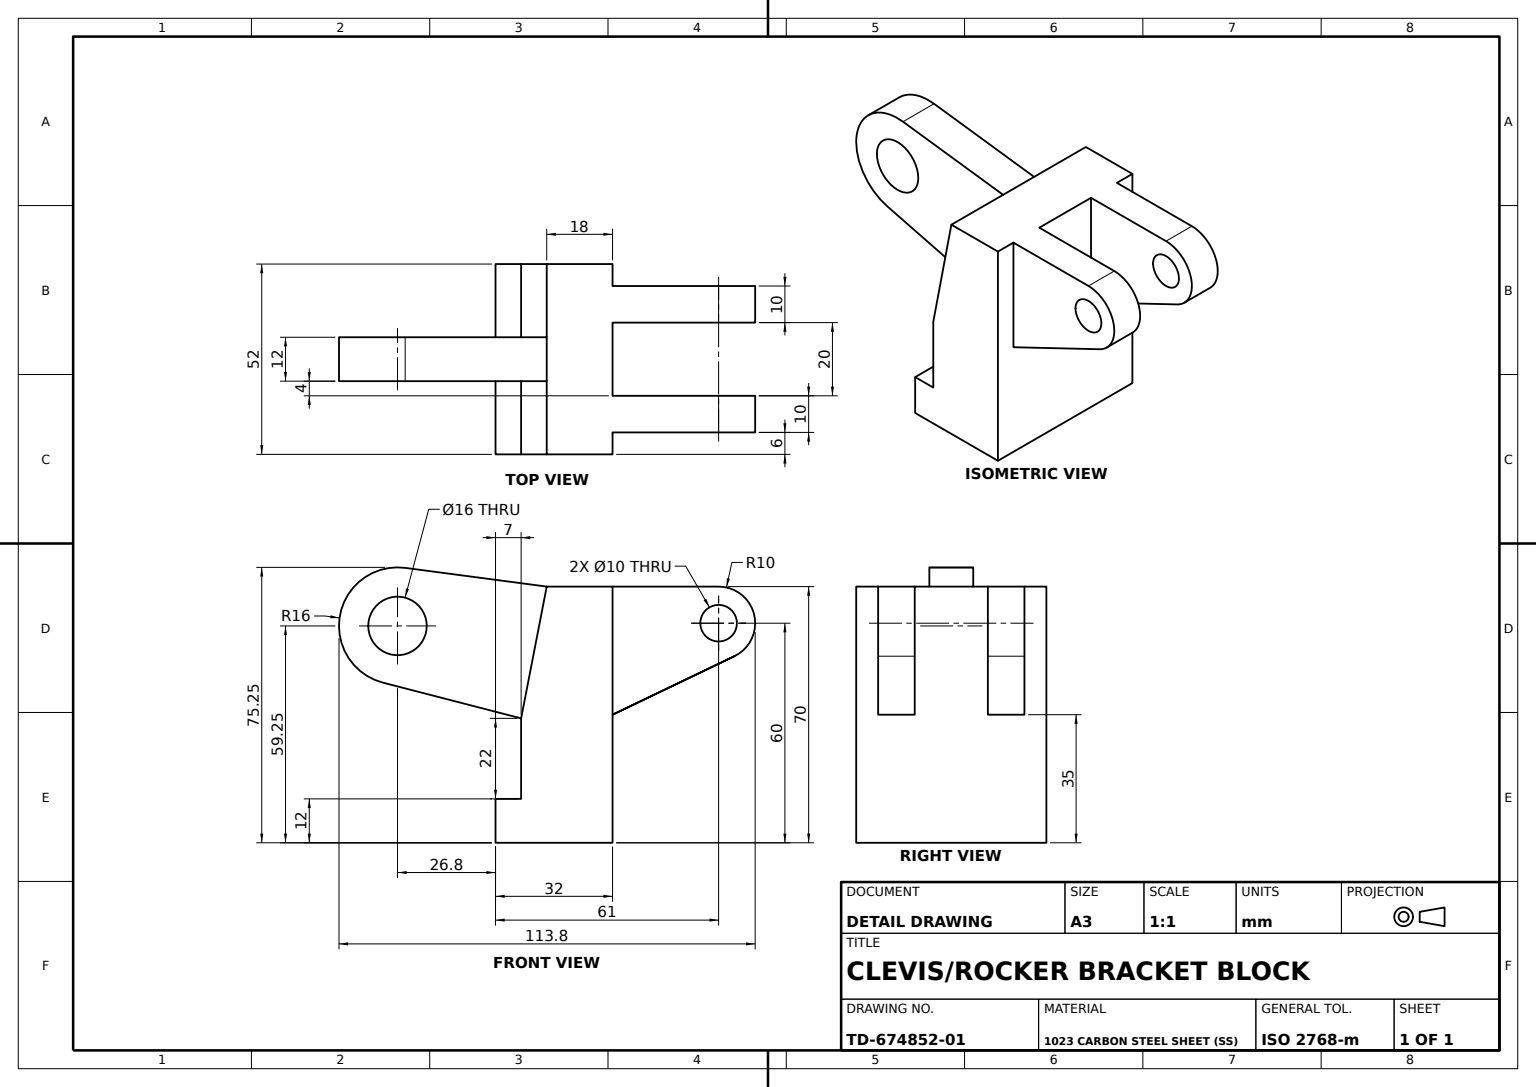
from build123d import *

# Parameters (mm, degrees)
BASE_BLOCK_SKETCH_W = 32
BASE_BLOCK_SKETCH_H = 12
BASE_BLOCK_DEPTH    = 52
UPRIGHT_BODY_DEPTH  = 52
CLEVIS_LUG_SKETCH_R = 5
CLEVIS_LUG_DEPTH    = 10
PIVOT_ARM_SKETCH_R  = 8
PIVOT_ARM_DEPTH     = 6


with BuildPart() as part:
    # Base Block Sketch → Base Block (new body)
    with BuildSketch(Plane.XY):
        with Locations((16, 6)):
            Rectangle(BASE_BLOCK_SKETCH_W, BASE_BLOCK_SKETCH_H)
    extrude(amount=BASE_BLOCK_DEPTH)

    # Upright Profile Sketch → Upright Body (add)
    with BuildSketch(Plane.XY.offset(52)):
        Polygon((32, 12), (32, 70), (14, 70), (7, 34), (7, 12), align=None)
    extrude(amount=-UPRIGHT_BODY_DEPTH)

    # Clevis Lug Sketch → Clevis Lug (add)
    with BuildSketch(Plane.XY.offset(6)):
        with BuildLine():
            Line((32, 70), (61, 70))
            ThreePointArc((61, 70), (70.751033946, 62.217506931), (65.324597071, 50.983467397))
            Line((65.324597071, 50.983467397), (32, 35))
            Line((32, 35), (32, 70))
        make_face()
        with Locations((61, 60)):
            Circle(CLEVIS_LUG_SKETCH_R, mode=Mode.SUBTRACT)
    clevis_lug = extrude(amount=CLEVIS_LUG_DEPTH)

    # Clevis Lug Mirror: Clevis Lug across plane
    add(clevis_lug.mirror(Plane.XY.offset(26)))

    # Pivot Arm Sketch → Pivot Arm (add, symmetric)
    with BuildSketch(Plane.XY.offset(26)):
        with BuildLine():
            Line((14, 70), (-24.705108972, 75.115128486))
            ThreePointArc((-24.705108972, 75.115128486), (-42.507231042, 62.306961592), (-30.8017068, 43.761196803))
            Line((-30.8017068, 43.761196803), (7, 34))
            Line((7, 34), (14, 70))
        make_face()
        with Locations((-26.801384807, 59.253047046)):
            Circle(PIVOT_ARM_SKETCH_R, mode=Mode.SUBTRACT)
    extrude(amount=PIVOT_ARM_DEPTH, both=True)


solid = part.part
